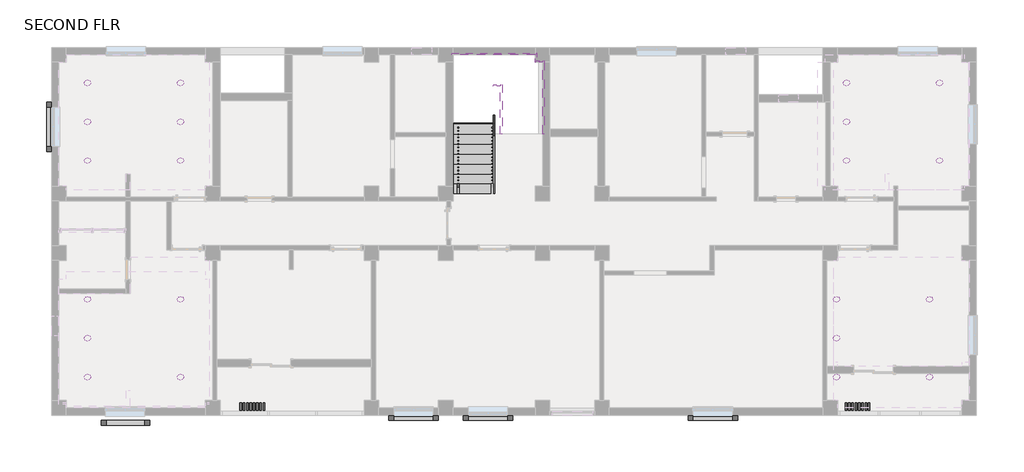
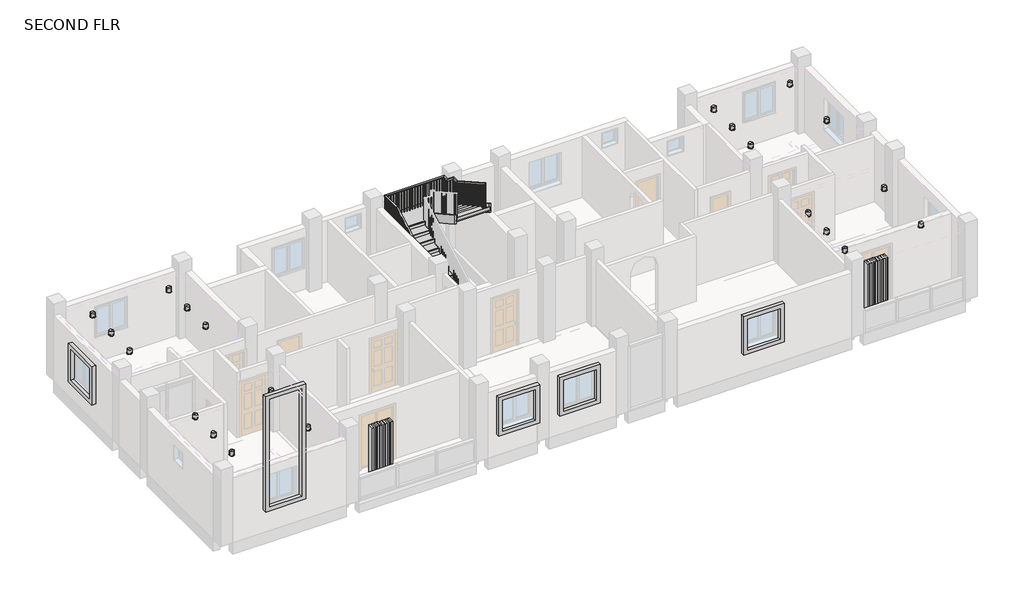
# One storey, part 5 of 5: 21 light fixtures, 8 members, 7 proxies, 1 railing, 1 stair flight.
"""IFC4 building model written with IfcOpenShell, lengths in millimetres."""

from ifc_helpers import new_model, si_unit, frame, origin, place, context, project, spatial, polyline, outline, extrude, faceted_brep, transform, mapped, element, save
from components import generic_models_13_generic_models_7_57cb182b, generic_models_17_generic_models_17_4194431e, generic_models_2_generic_models_2_798ec4a6, generic_models_21_generic_models_21_07dc1754, light_modern_pendant_14774_baffle_cc9af11b, light_modern_pendant_14774_baffle_b3430626, stair_flight_991562f7

model = new_model("IFC4")

# Units and contexts
model_context = context("Model", 3, world=origin())
ifc_project = project(units=[si_unit("LENGTHUNIT", "METRE", prefix="MILLI")], contexts=[model_context])

# Site, building, storey
site = spatial("IfcSite", under=ifc_project)
building = spatial("IfcBuilding", under=site)
storey = spatial("IfcBuildingStorey", under=building, Name="SECOND FLR", Elevation=6400.8)

# Proxies
placement = place(None, origin())
generic_models_13_generic_models_7_shape = generic_models_13_generic_models_7_57cb182b(model_context)
element("IfcBuildingElementProxy", 1, Name="Generic Models 13 : Generic Models 7", ObjectType="Generic Models 13 : Generic Models 7", at=placement, inside=storey, context=model_context, shape_type="MappedRepresentation", body=[
    mapped(generic_models_13_generic_models_7_shape, transform((18592.8, 152.4, 0.0), x_axis=(1.0, 0.0, 0.0), y_axis=(0.0, 1.0, 0.0), z_axis=(0.0, 0.0, 1.0))),
])
generic_models_17_generic_models_17_shape = generic_models_17_generic_models_17_4194431e(model_context)
element("IfcBuildingElementProxy", 2, Name="Generic Models 18 : Generic Models 17", ObjectType="Generic Models 18 : Generic Models 17", at=placement, inside=storey, context=model_context, shape_type="MappedRepresentation", body=[
    mapped(generic_models_17_generic_models_17_shape, transform((0.0, 0.0, -3048.0), x_axis=(1.0, 0.0, 0.0), y_axis=(0.0, 1.0, 0.0), z_axis=(0.0, 0.0, 1.0))),
])
generic_models_2_generic_models_2_shape = generic_models_2_generic_models_2_798ec4a6(model_context)
element("IfcBuildingElementProxy", 3, Name="Generic Models 2 : Generic Models 2", ObjectType="Generic Models 2 : Generic Models 2", at=placement, inside=storey, context=model_context, shape_type="MappedRepresentation", body=[
    mapped(generic_models_2_generic_models_2_shape, transform((0.0, 0.0, 0.0), x_axis=(1.0, 0.0, 0.0), y_axis=(0.0, 1.0, 0.0), z_axis=(0.0, 0.0, 1.0))),
])
generic_models_21_generic_models_21_shape = generic_models_21_generic_models_21_07dc1754(model_context)
element("IfcBuildingElementProxy", 4, Name="Generic Models 22 : Generic Models 21", ObjectType="Generic Models 22 : Generic Models 21", at=placement, inside=storey, context=model_context, shape_type="MappedRepresentation", body=[
    mapped(generic_models_21_generic_models_21_shape, transform((0.0, 0.0, -3048.0), x_axis=(1.0, 0.0, 0.0), y_axis=(0.0, 1.0, 0.0), z_axis=(0.0, 0.0, 1.0))),
])
element("IfcBuildingElementProxy", 5, Name="Generic Models 26 : Generic Models 21", ObjectType="Generic Models 26 : Generic Models 21", at=placement, inside=storey, context=model_context, shape_type="MappedRepresentation", body=[
    mapped(generic_models_21_generic_models_21_shape, transform((-6905.3372689, 0.0, -3048.0), x_axis=(1.0, 0.0, 0.0), y_axis=(0.0, 1.0, 0.0), z_axis=(0.0, 0.0, 1.0))),
])
element("IfcBuildingElementProxy", 6, Name="Generic Models 30 : Generic Models 21", ObjectType="Generic Models 30 : Generic Models 21", at=placement, inside=storey, context=model_context, shape_type="MappedRepresentation", body=[
    mapped(generic_models_21_generic_models_21_shape, transform((-9191.3372689, 0.0, -3048.0), x_axis=(1.0, 0.0, 0.0), y_axis=(0.0, 1.0, 0.0), z_axis=(0.0, 0.0, 1.0))),
])
element("IfcBuildingElementProxy", 7, Name="Generic Models 7 : Generic Models 7", ObjectType="Generic Models 7 : Generic Models 7", at=placement, inside=storey, context=model_context, shape_type="MappedRepresentation", body=[
    mapped(generic_models_13_generic_models_7_shape, transform((0.0, 152.4, 0.0), x_axis=(1.0, 0.0, 0.0), y_axis=(0.0, 1.0, 0.0), z_axis=(0.0, 0.0, 1.0))),
])

# Light fixtures
light_modern_pendant_14774_baffle_shape = light_modern_pendant_14774_baffle_cc9af11b(model_context)
element("IfcLightFixture", 8, ObjectType="LIGHT_-_MODERN_PENDANT_14774 : Baffle", at=placement, inside=storey, context=model_context, shape_type="MappedRepresentation", body=[
    mapped(light_modern_pendant_14774_baffle_shape, transform((-14269.0456086, -897.3794704, 6527.8), x_axis=(1.0, 0.0, 0.0), y_axis=(0.0, 1.0, 0.0), z_axis=(0.0, 0.0, 1.0))),
])
element("IfcLightFixture", 9, ObjectType="LIGHT_-_MODERN_PENDANT_14774 : Baffle", at=placement, inside=storey, context=model_context, shape_type="MappedRepresentation", body=[
    mapped(light_modern_pendant_14774_baffle_shape, transform((-14269.0456086, -3284.9794704, 6527.8), x_axis=(1.0, 0.0, 0.0), y_axis=(0.0, 1.0, 0.0), z_axis=(0.0, 0.0, 1.0))),
])
element("IfcLightFixture", 10, ObjectType="LIGHT_-_MODERN_PENDANT_14774 : Baffle", at=placement, inside=storey, context=model_context, shape_type="MappedRepresentation", body=[
    mapped(light_modern_pendant_14774_baffle_shape, transform((-14269.0456086, -2091.1794704, 6527.8), x_axis=(1.0, 0.0, 0.0), y_axis=(0.0, 1.0, 0.0), z_axis=(0.0, 0.0, 1.0))),
])
element("IfcLightFixture", 11, ObjectType="LIGHT_-_MODERN_PENDANT_14774 : Baffle", at=placement, inside=storey, context=model_context, shape_type="MappedRepresentation", body=[
    mapped(light_modern_pendant_14774_baffle_shape, transform((9048.1543914, -897.3794704, 6527.8), x_axis=(1.0, 0.0, 0.0), y_axis=(0.0, 1.0, 0.0), z_axis=(0.0, 0.0, 1.0))),
])
element("IfcLightFixture", 12, ObjectType="LIGHT_-_MODERN_PENDANT_14774 : Baffle", at=placement, inside=storey, context=model_context, shape_type="MappedRepresentation", body=[
    mapped(light_modern_pendant_14774_baffle_shape, transform((9048.1543914, -3284.9794704, 6527.8), x_axis=(1.0, 0.0, 0.0), y_axis=(0.0, 1.0, 0.0), z_axis=(0.0, 0.0, 1.0))),
])
element("IfcLightFixture", 13, ObjectType="LIGHT_-_MODERN_PENDANT_14774 : Baffle", at=placement, inside=storey, context=model_context, shape_type="MappedRepresentation", body=[
    mapped(light_modern_pendant_14774_baffle_shape, transform((9048.1543914, -2091.1794704, 6527.8), x_axis=(1.0, 0.0, 0.0), y_axis=(0.0, 1.0, 0.0), z_axis=(0.0, 0.0, 1.0))),
])
element("IfcLightFixture", 14, ObjectType="LIGHT_-_MODERN_PENDANT_14774 : Baffle", at=placement, inside=storey, context=model_context, shape_type="MappedRepresentation", body=[
    mapped(light_modern_pendant_14774_baffle_shape, transform((-14269.0456086, -7552.1794704, 6527.8), x_axis=(1.0, 0.0, 0.0), y_axis=(0.0, 1.0, 0.0), z_axis=(0.0, 0.0, 1.0))),
])
element("IfcLightFixture", 15, ObjectType="LIGHT_-_MODERN_PENDANT_14774 : Baffle", at=placement, inside=storey, context=model_context, shape_type="MappedRepresentation", body=[
    mapped(light_modern_pendant_14774_baffle_shape, transform((-14269.0456086, -9939.7794704, 6527.8), x_axis=(1.0, 0.0, 0.0), y_axis=(0.0, 1.0, 0.0), z_axis=(0.0, 0.0, 1.0))),
])
element("IfcLightFixture", 16, ObjectType="LIGHT_-_MODERN_PENDANT_14774 : Baffle", at=placement, inside=storey, context=model_context, shape_type="MappedRepresentation", body=[
    mapped(light_modern_pendant_14774_baffle_shape, transform((-14269.0456086, -8745.9794704, 6527.8), x_axis=(1.0, 0.0, 0.0), y_axis=(0.0, 1.0, 0.0), z_axis=(0.0, 0.0, 1.0))),
])
element("IfcLightFixture", 17, ObjectType="LIGHT_-_MODERN_PENDANT_14774 : Baffle", at=placement, inside=storey, context=model_context, shape_type="MappedRepresentation", body=[
    mapped(light_modern_pendant_14774_baffle_shape, transform((8743.3543914, -7552.1794704, 6527.8), x_axis=(1.0, 0.0, 0.0), y_axis=(0.0, 1.0, 0.0), z_axis=(0.0, 0.0, 1.0))),
])
element("IfcLightFixture", 18, ObjectType="LIGHT_-_MODERN_PENDANT_14774 : Baffle", at=placement, inside=storey, context=model_context, shape_type="MappedRepresentation", body=[
    mapped(light_modern_pendant_14774_baffle_shape, transform((8743.3543914, -9939.7794704, 6527.8), x_axis=(1.0, 0.0, 0.0), y_axis=(0.0, 1.0, 0.0), z_axis=(0.0, 0.0, 1.0))),
])
element("IfcLightFixture", 19, ObjectType="LIGHT_-_MODERN_PENDANT_14774 : Baffle", at=placement, inside=storey, context=model_context, shape_type="MappedRepresentation", body=[
    mapped(light_modern_pendant_14774_baffle_shape, transform((8743.3543914, -8745.9794704, 6527.8), x_axis=(1.0, 0.0, 0.0), y_axis=(0.0, 1.0, 0.0), z_axis=(0.0, 0.0, 1.0))),
])
light_modern_pendant_14774_baffle_2_shape = light_modern_pendant_14774_baffle_b3430626(model_context)
element("IfcLightFixture", 20, ObjectType="LIGHT_-_MODERN_PENDANT_14774 : Baffle", at=placement, inside=storey, context=model_context, shape_type="MappedRepresentation", body=[
    mapped(light_modern_pendant_14774_baffle_2_shape, transform((-11411.5456086, -897.3794704, 6527.8), x_axis=(-1.0, 0.0, 0.0), y_axis=(0.0, -1.0, 0.0), z_axis=(0.0, 0.0, 1.0))),
])
element("IfcLightFixture", 21, ObjectType="LIGHT_-_MODERN_PENDANT_14774 : Baffle", at=placement, inside=storey, context=model_context, shape_type="MappedRepresentation", body=[
    mapped(light_modern_pendant_14774_baffle_2_shape, transform((-11411.5456086, -3284.9794704, 6527.8), x_axis=(-1.0, 0.0, 0.0), y_axis=(0.0, -1.0, 0.0), z_axis=(0.0, 0.0, 1.0))),
])
element("IfcLightFixture", 22, ObjectType="LIGHT_-_MODERN_PENDANT_14774 : Baffle", at=placement, inside=storey, context=model_context, shape_type="MappedRepresentation", body=[
    mapped(light_modern_pendant_14774_baffle_2_shape, transform((-11411.5456086, -2091.1794704, 6527.8), x_axis=(-1.0, 0.0, 0.0), y_axis=(0.0, -1.0, 0.0), z_axis=(0.0, 0.0, 1.0))),
])
element("IfcLightFixture", 23, ObjectType="LIGHT_-_MODERN_PENDANT_14774 : Baffle", at=placement, inside=storey, context=model_context, shape_type="MappedRepresentation", body=[
    mapped(light_modern_pendant_14774_baffle_2_shape, transform((11905.6543914, -897.3794704, 6527.8), x_axis=(-1.0, 0.0, 0.0), y_axis=(0.0, -1.0, 0.0), z_axis=(0.0, 0.0, 1.0))),
])
element("IfcLightFixture", 24, ObjectType="LIGHT_-_MODERN_PENDANT_14774 : Baffle", at=placement, inside=storey, context=model_context, shape_type="MappedRepresentation", body=[
    mapped(light_modern_pendant_14774_baffle_2_shape, transform((11905.6543914, -3284.9794704, 6527.8), x_axis=(-1.0, 0.0, 0.0), y_axis=(0.0, -1.0, 0.0), z_axis=(0.0, 0.0, 1.0))),
])
element("IfcLightFixture", 25, ObjectType="LIGHT_-_MODERN_PENDANT_14774 : Baffle", at=placement, inside=storey, context=model_context, shape_type="MappedRepresentation", body=[
    mapped(light_modern_pendant_14774_baffle_2_shape, transform((-11411.5456086, -7552.1794704, 6527.8), x_axis=(-1.0, 0.0, 0.0), y_axis=(0.0, -1.0, 0.0), z_axis=(0.0, 0.0, 1.0))),
])
element("IfcLightFixture", 26, ObjectType="LIGHT_-_MODERN_PENDANT_14774 : Baffle", at=placement, inside=storey, context=model_context, shape_type="MappedRepresentation", body=[
    mapped(light_modern_pendant_14774_baffle_2_shape, transform((-11411.5456086, -9939.7794704, 6527.8), x_axis=(-1.0, 0.0, 0.0), y_axis=(0.0, -1.0, 0.0), z_axis=(0.0, 0.0, 1.0))),
])
element("IfcLightFixture", 27, ObjectType="LIGHT_-_MODERN_PENDANT_14774 : Baffle", at=placement, inside=storey, context=model_context, shape_type="MappedRepresentation", body=[
    mapped(light_modern_pendant_14774_baffle_2_shape, transform((11600.8543914, -7552.1794704, 6527.8), x_axis=(-1.0, 0.0, 0.0), y_axis=(0.0, -1.0, 0.0), z_axis=(0.0, 0.0, 1.0))),
])
element("IfcLightFixture", 28, ObjectType="LIGHT_-_MODERN_PENDANT_14774 : Baffle", at=placement, inside=storey, context=model_context, shape_type="MappedRepresentation", body=[
    mapped(light_modern_pendant_14774_baffle_2_shape, transform((11600.8543914, -9939.7794704, 6527.8), x_axis=(-1.0, 0.0, 0.0), y_axis=(0.0, -1.0, 0.0), z_axis=(0.0, 0.0, 1.0))),
])

# Members
element("IfcMember", 29, ObjectType="Stringer - 2\" Width", at=placement, inside=storey, context=model_context, shape_type="SweptSolid", body=[
    extrude(outline(polyline([(-4300.9794704, 6400.8), (-4300.9794704, 6608.3983948), (-879.896581, 8509.0), (-252.2749676, 8509.0), (-4047.0349676, 6400.8), (-4300.9794704, 6400.8)])), frame((-3080.3456086, 0.0, 0.0), z_axis=(1.0, 0.0, 0.0), x_axis=(0.0, 1.0, 0.0)), (0.0, 0.0, 1.0), 50.8),
])
element("IfcMember", 30, ObjectType="Stringer - 2\" Width", at=placement, inside=storey, context=model_context, shape_type="SweptSolid", body=[
    extrude(outline(polyline([(-3080.3456086, -33.7794704), (-3080.3456086, 17.0205296), (-467.6083398, 17.0205296), (-518.4083398, -33.7794704), (-3080.3456086, -33.7794704)])), frame((0.0, 0.0, 8204.2), z_axis=(0.0, 0.0, 1.0), x_axis=(1.0, 0.0, 0.0)), (0.0, 0.0, 1.0), 304.8),
])
element("IfcMember", 31, ObjectType="Stringer - 2\" Width", at=placement, inside=storey, context=model_context, shape_type="SweptSolid", body=[
    extrude(outline(polyline([(-518.4083398, -33.7794704), (-467.6083398, 17.0205296), (-467.6083398, -211.5794704), (-518.4083398, -262.3794704), (-518.4083398, -33.7794704)])), frame((0.0, 0.0, 8204.2), z_axis=(0.0, 0.0, 1.0), x_axis=(1.0, 0.0, 0.0)), (0.0, 0.0, 1.0), 304.8),
])
element("IfcMember", 32, ObjectType="Stringer - 2\" Width", at=placement, inside=storey, context=model_context, shape_type="SweptSolid", body=[
    extrude(outline(polyline([(-518.4083398, -262.3794704), (-467.6083398, -211.5794704), (-289.8083398, -211.5794704), (-289.8083398, -262.3794704), (-518.4083398, -262.3794704)])), frame((0.0, 0.0, 8204.2), z_axis=(0.0, 0.0, 1.0), x_axis=(1.0, 0.0, 0.0)), (0.0, 0.0, 1.0), 304.8),
])
element("IfcMember", 33, ObjectType="Stringer - 2\" Width", at=placement, inside=storey, context=model_context, shape_type="SweptSolid", body=[
    extrude(outline(polyline([(-211.5794704, 8231.1761726), (-211.5794704, 8204.2), (-790.6439732, 8204.2), (-2472.1794704, 9138.3863873), (-2472.1794704, 9487.0650614), (-211.5794704, 8231.1761726)])), frame((-289.8083398, 0.0, 0.0), z_axis=(1.0, 0.0, 0.0), x_axis=(0.0, 1.0, 0.0)), (0.0, 0.0, 1.0), 50.8),
])
element("IfcMember", 34, ObjectType="Stringer - 2\" Width", at=placement, inside=storey, context=model_context, shape_type="SweptSolid", body=[
    extrude(outline(polyline([(-4300.9794704, 6400.8), (-4300.9794704, 6608.3983948), (-998.9794704, 8442.8428392), (-998.9794704, 8094.1641651), (-4047.0349676, 6400.8), (-4300.9794704, 6400.8)])), frame((-1810.3456086, 0.0, 0.0), z_axis=(1.0, 0.0, 0.0), x_axis=(0.0, 1.0, 0.0)), (0.0, 0.0, 1.0), 50.8),
])
element("IfcMember", 35, ObjectType="Stringer - 2\" Width", at=placement, inside=storey, context=model_context, shape_type="SweptSolid", body=[
    extrude(outline(polyline([(-1810.3456086, -998.9794704), (-1810.3456086, -948.1794704), (-1585.2083398, -948.1794704), (-1585.2083398, -998.9794704), (-1810.3456086, -998.9794704)])), frame((0.0, 0.0, 8204.2), z_axis=(0.0, 0.0, 1.0), x_axis=(1.0, 0.0, 0.0)), (0.0, 0.0, 1.0), 304.8),
])
element("IfcMember", 36, ObjectType="Stringer - 2\" Width", at=placement, inside=storey, context=model_context, shape_type="SweptSolid", body=[
    extrude(outline(polyline([(-948.1794704, 8640.3983948), (-948.1794704, 8291.7197207), (-2472.1794704, 9138.3863873), (-2472.1794704, 9487.0650614), (-948.1794704, 8640.3983948)])), frame((-1585.2083398, 0.0, 0.0), z_axis=(1.0, 0.0, 0.0), x_axis=(0.0, 1.0, 0.0)), (0.0, 0.0, 1.0), 50.8),
])

# Railing
element("IfcRailing", 37, ObjectType="Handrail - Rectangular", at=placement, inside=storey, context=model_context, shape_type="SolidModel", body=[
    faceted_brep([(-2902.5456086, -4300.9794704, 7484.5333333), (-2902.5456086, -4300.9794704, 7426.420221), (-2851.7456086, -4300.9794704, 7426.420221), (-2851.7456086, -4300.9794704, 7484.5333333), (-2902.5456086, -948.1794704, 9347.2), (-2902.5456086, -935.0158682, 9296.4), (-2851.7456086, -935.0158682, 9296.4), (-2851.7456086, -948.1794704, 9347.2), (-2902.5456086, -160.7794704, 9347.2), (-2902.5456086, -160.7794704, 9296.4), (-2851.7456086, -211.5794704, 9296.4), (-2851.7456086, -211.5794704, 9347.2), (-645.4083398, -160.7794704, 9347.2), (-645.4083398, -160.7794704, 9296.4), (-696.2083398, -211.5794704, 9296.4), (-696.2083398, -211.5794704, 9347.2), (-645.4083398, -389.3794704, 9347.2), (-645.4083398, -389.3794704, 9296.4), (-696.2083398, -440.1794704, 9296.4), (-696.2083398, -440.1794704, 9347.2), (-416.8083398, -389.3794704, 9347.2), (-416.8083398, -389.3794704, 9296.4), (-467.6083398, -440.1794704, 9296.4), (-467.6083398, -440.1794704, 9347.2), (-416.8083398, -643.3794704, 9347.2), (-416.8083398, -656.5430727, 9296.4), (-467.6083398, -656.5430727, 9296.4), (-467.6083398, -643.3794704, 9347.2), (-416.8083398, -2472.1794704, 10363.2), (-467.6083398, -2472.1794704, 10363.2), (-467.6083398, -2472.1794704, 10305.0868876), (-416.8083398, -2472.1794704, 10305.0868876)], [[[0, 1, 2, 3]], [[1, 0, 4, 5]], [[2, 1, 5, 6]], [[3, 2, 6, 7]], [[0, 3, 7, 4]], [[5, 4, 8, 9]], [[6, 5, 9, 10]], [[7, 6, 10, 11]], [[4, 7, 11, 8]], [[9, 8, 12, 13]], [[10, 9, 13, 14]], [[11, 10, 14, 15]], [[8, 11, 15, 12]], [[13, 12, 16, 17]], [[14, 13, 17, 18]], [[15, 14, 18, 19]], [[12, 15, 19, 16]], [[17, 16, 20, 21]], [[18, 17, 21, 22]], [[19, 18, 22, 23]], [[16, 19, 23, 20]], [[21, 20, 24, 25]], [[22, 21, 25, 26]], [[23, 22, 26, 27]], [[20, 23, 27, 24]], [[28, 29, 30, 31]], [[25, 24, 28, 31]], [[26, 25, 31, 30]], [[27, 26, 30, 29]], [[24, 27, 29, 28]]]),
    extrude(outline(polyline([(-2437.2544704, 10285.6841099), (-2437.2544704, 9279.4666667), (-2456.3044704, 9279.4666667), (-2456.3044704, 10296.2674432), (-2437.2544704, 10285.6841099)])), frame((-451.7333398, 0.0, 0.0), z_axis=(1.0, 0.0, 0.0), x_axis=(0.0, 1.0, 0.0)), (0.0, 0.0, 1.0), 19.05),
    extrude(outline(polyline([(-2335.6544704, 10229.2396654), (-2335.6544704, 9279.4666667), (-2354.7044704, 9279.4666667), (-2354.7044704, 10239.8229988), (-2335.6544704, 10229.2396654)])), frame((-451.7333398, 0.0, 0.0), z_axis=(1.0, 0.0, 0.0), x_axis=(0.0, 1.0, 0.0)), (0.0, 0.0, 1.0), 19.05),
    extrude(outline(polyline([(-2234.0544704, 10172.795221), (-2234.0544704, 9279.4666667), (-2253.1044704, 9279.4666667), (-2253.1044704, 10183.3785543), (-2234.0544704, 10172.795221)])), frame((-451.7333398, 0.0, 0.0), z_axis=(1.0, 0.0, 0.0), x_axis=(0.0, 1.0, 0.0)), (0.0, 0.0, 1.0), 19.05),
    extrude(outline(polyline([(-2132.4544704, 10116.3507765), (-2132.4544704, 9110.1333333), (-2151.5044704, 9110.1333333), (-2151.5044704, 10126.9341099), (-2132.4544704, 10116.3507765)])), frame((-451.7333398, 0.0, 0.0), z_axis=(1.0, 0.0, 0.0), x_axis=(0.0, 1.0, 0.0)), (0.0, 0.0, 1.0), 19.05),
    extrude(outline(polyline([(-2030.8544704, 10059.9063321), (-2030.8544704, 9110.1333333), (-2049.9044704, 9110.1333333), (-2049.9044704, 10070.4896654), (-2030.8544704, 10059.9063321)])), frame((-451.7333398, 0.0, 0.0), z_axis=(1.0, 0.0, 0.0), x_axis=(0.0, 1.0, 0.0)), (0.0, 0.0, 1.0), 19.05),
    extrude(outline(polyline([(-1929.2544704, 10003.4618876), (-1929.2544704, 9110.1333333), (-1948.3044704, 9110.1333333), (-1948.3044704, 10014.045221), (-1929.2544704, 10003.4618876)])), frame((-451.7333398, 0.0, 0.0), z_axis=(1.0, 0.0, 0.0), x_axis=(0.0, 1.0, 0.0)), (0.0, 0.0, 1.0), 19.05),
    extrude(outline(polyline([(-1827.6544704, 9947.0174432), (-1827.6544704, 8940.8), (-1846.7044704, 8940.8), (-1846.7044704, 9957.6007765), (-1827.6544704, 9947.0174432)])), frame((-451.7333398, 0.0, 0.0), z_axis=(1.0, 0.0, 0.0), x_axis=(0.0, 1.0, 0.0)), (0.0, 0.0, 1.0), 19.05),
    extrude(outline(polyline([(-1726.0544704, 9890.5729988), (-1726.0544704, 8940.8), (-1745.1044704, 8940.8), (-1745.1044704, 9901.1563321), (-1726.0544704, 9890.5729988)])), frame((-451.7333398, 0.0, 0.0), z_axis=(1.0, 0.0, 0.0), x_axis=(0.0, 1.0, 0.0)), (0.0, 0.0, 1.0), 19.05),
    extrude(outline(polyline([(-1624.4544704, 9834.1285543), (-1624.4544704, 8940.8), (-1643.5044704, 8940.8), (-1643.5044704, 9844.7118876), (-1624.4544704, 9834.1285543)])), frame((-451.7333398, 0.0, 0.0), z_axis=(1.0, 0.0, 0.0), x_axis=(0.0, 1.0, 0.0)), (0.0, 0.0, 1.0), 19.05),
    extrude(outline(polyline([(-1522.8544704, 9777.6841099), (-1522.8544704, 8771.4666667), (-1541.9044704, 8771.4666667), (-1541.9044704, 9788.2674432), (-1522.8544704, 9777.6841099)])), frame((-451.7333398, 0.0, 0.0), z_axis=(1.0, 0.0, 0.0), x_axis=(0.0, 1.0, 0.0)), (0.0, 0.0, 1.0), 19.05),
    extrude(outline(polyline([(-1421.2544704, 9721.2396654), (-1421.2544704, 8771.4666667), (-1440.3044704, 8771.4666667), (-1440.3044704, 9731.8229988), (-1421.2544704, 9721.2396654)])), frame((-451.7333398, 0.0, 0.0), z_axis=(1.0, 0.0, 0.0), x_axis=(0.0, 1.0, 0.0)), (0.0, 0.0, 1.0), 19.05),
    extrude(outline(polyline([(-1319.6544704, 9664.795221), (-1319.6544704, 8771.4666667), (-1338.7044704, 8771.4666667), (-1338.7044704, 9675.3785543), (-1319.6544704, 9664.795221)])), frame((-451.7333398, 0.0, 0.0), z_axis=(1.0, 0.0, 0.0), x_axis=(0.0, 1.0, 0.0)), (0.0, 0.0, 1.0), 19.05),
    extrude(outline(polyline([(-1218.0544704, 9608.3507765), (-1218.0544704, 8602.1333333), (-1237.1044704, 8602.1333333), (-1237.1044704, 9618.9341099), (-1218.0544704, 9608.3507765)])), frame((-451.7333398, 0.0, 0.0), z_axis=(1.0, 0.0, 0.0), x_axis=(0.0, 1.0, 0.0)), (0.0, 0.0, 1.0), 19.05),
    extrude(outline(polyline([(-1116.4544704, 9551.9063321), (-1116.4544704, 8602.1333333), (-1135.5044704, 8602.1333333), (-1135.5044704, 9562.4896654), (-1116.4544704, 9551.9063321)])), frame((-451.7333398, 0.0, 0.0), z_axis=(1.0, 0.0, 0.0), x_axis=(0.0, 1.0, 0.0)), (0.0, 0.0, 1.0), 19.05),
    extrude(outline(polyline([(-1014.8544704, 9495.4618876), (-1014.8544704, 8602.1333333), (-1033.9044704, 8602.1333333), (-1033.9044704, 9506.045221), (-1014.8544704, 9495.4618876)])), frame((-451.7333398, 0.0, 0.0), z_axis=(1.0, 0.0, 0.0), x_axis=(0.0, 1.0, 0.0)), (0.0, 0.0, 1.0), 19.05),
    extrude(outline(polyline([(-913.2544704, 9439.0174432), (-913.2544704, 8432.8), (-932.3044704, 8432.8), (-932.3044704, 9449.6007765), (-913.2544704, 9439.0174432)])), frame((-451.7333398, 0.0, 0.0), z_axis=(1.0, 0.0, 0.0), x_axis=(0.0, 1.0, 0.0)), (0.0, 0.0, 1.0), 19.05),
    extrude(outline(polyline([(-811.6544704, 9382.5729988), (-811.6544704, 8432.8), (-830.7044704, 8432.8), (-830.7044704, 9393.1563321), (-811.6544704, 9382.5729988)])), frame((-451.7333398, 0.0, 0.0), z_axis=(1.0, 0.0, 0.0), x_axis=(0.0, 1.0, 0.0)), (0.0, 0.0, 1.0), 19.05),
    extrude(outline(polyline([(-710.0544704, 9326.1285543), (-710.0544704, 8432.8), (-729.1044704, 8432.8), (-729.1044704, 9336.7118876), (-710.0544704, 9326.1285543)])), frame((-451.7333398, 0.0, 0.0), z_axis=(1.0, 0.0, 0.0), x_axis=(0.0, 1.0, 0.0)), (0.0, 0.0, 1.0), 19.05),
    extrude(outline(polyline([(-432.6833398, -608.4544704), (-432.6833398, -627.5044704), (-451.7333398, -627.5044704), (-451.7333398, -608.4544704), (-432.6833398, -608.4544704)])), frame((0.0, 0.0, 8432.8), z_axis=(0.0, 0.0, 1.0), x_axis=(1.0, 0.0, 0.0)), (0.0, 0.0, 1.0), 863.6),
    extrude(outline(polyline([(-432.6833398, -506.8544704), (-432.6833398, -525.9044704), (-451.7333398, -525.9044704), (-451.7333398, -506.8544704), (-432.6833398, -506.8544704)])), frame((0.0, 0.0, 8432.8), z_axis=(0.0, 0.0, 1.0), x_axis=(1.0, 0.0, 0.0)), (0.0, 0.0, 1.0), 863.6),
    extrude(outline(polyline([(-477.1333398, -405.2544704), (-458.0833398, -405.2544704), (-458.0833398, -424.3044704), (-477.1333398, -424.3044704), (-477.1333398, -405.2544704)])), frame((0.0, 0.0, 8432.8), z_axis=(0.0, 0.0, 1.0), x_axis=(1.0, 0.0, 0.0)), (0.0, 0.0, 1.0), 863.6),
    extrude(outline(polyline([(-578.7333398, -405.2544704), (-559.6833398, -405.2544704), (-559.6833398, -424.3044704), (-578.7333398, -424.3044704), (-578.7333398, -405.2544704)])), frame((0.0, 0.0, 8432.8), z_axis=(0.0, 0.0, 1.0), x_axis=(1.0, 0.0, 0.0)), (0.0, 0.0, 1.0), 863.6),
    extrude(outline(polyline([(-661.2833398, -379.8544704), (-661.2833398, -398.9044704), (-680.3333398, -398.9044704), (-680.3333398, -379.8544704), (-661.2833398, -379.8544704)])), frame((0.0, 0.0, 8432.8), z_axis=(0.0, 0.0, 1.0), x_axis=(1.0, 0.0, 0.0)), (0.0, 0.0, 1.0), 863.6),
    extrude(outline(polyline([(-661.2833398, -278.2544704), (-661.2833398, -297.3044704), (-680.3333398, -297.3044704), (-680.3333398, -278.2544704), (-661.2833398, -278.2544704)])), frame((0.0, 0.0, 8432.8), z_axis=(0.0, 0.0, 1.0), x_axis=(1.0, 0.0, 0.0)), (0.0, 0.0, 1.0), 863.6),
    extrude(outline(polyline([(-753.0706086, -176.6544704), (-734.0206086, -176.6544704), (-734.0206086, -195.7044704), (-753.0706086, -195.7044704), (-753.0706086, -176.6544704)])), frame((0.0, 0.0, 8432.8), z_axis=(0.0, 0.0, 1.0), x_axis=(1.0, 0.0, 0.0)), (0.0, 0.0, 1.0), 863.6),
    extrude(outline(polyline([(-854.6706086, -176.6544704), (-835.6206086, -176.6544704), (-835.6206086, -195.7044704), (-854.6706086, -195.7044704), (-854.6706086, -176.6544704)])), frame((0.0, 0.0, 8432.8), z_axis=(0.0, 0.0, 1.0), x_axis=(1.0, 0.0, 0.0)), (0.0, 0.0, 1.0), 863.6),
    extrude(outline(polyline([(-956.2706086, -176.6544704), (-937.2206086, -176.6544704), (-937.2206086, -195.7044704), (-956.2706086, -195.7044704), (-956.2706086, -176.6544704)])), frame((0.0, 0.0, 8432.8), z_axis=(0.0, 0.0, 1.0), x_axis=(1.0, 0.0, 0.0)), (0.0, 0.0, 1.0), 863.6),
    extrude(outline(polyline([(-1057.8706086, -176.6544704), (-1038.8206086, -176.6544704), (-1038.8206086, -195.7044704), (-1057.8706086, -195.7044704), (-1057.8706086, -176.6544704)])), frame((0.0, 0.0, 8432.8), z_axis=(0.0, 0.0, 1.0), x_axis=(1.0, 0.0, 0.0)), (0.0, 0.0, 1.0), 863.6),
    extrude(outline(polyline([(-1159.4706086, -176.6544704), (-1140.4206086, -176.6544704), (-1140.4206086, -195.7044704), (-1159.4706086, -195.7044704), (-1159.4706086, -176.6544704)])), frame((0.0, 0.0, 8432.8), z_axis=(0.0, 0.0, 1.0), x_axis=(1.0, 0.0, 0.0)), (0.0, 0.0, 1.0), 863.6),
    extrude(outline(polyline([(-1261.0706086, -176.6544704), (-1242.0206086, -176.6544704), (-1242.0206086, -195.7044704), (-1261.0706086, -195.7044704), (-1261.0706086, -176.6544704)])), frame((0.0, 0.0, 8432.8), z_axis=(0.0, 0.0, 1.0), x_axis=(1.0, 0.0, 0.0)), (0.0, 0.0, 1.0), 863.6),
    extrude(outline(polyline([(-1362.6706086, -176.6544704), (-1343.6206086, -176.6544704), (-1343.6206086, -195.7044704), (-1362.6706086, -195.7044704), (-1362.6706086, -176.6544704)])), frame((0.0, 0.0, 8432.8), z_axis=(0.0, 0.0, 1.0), x_axis=(1.0, 0.0, 0.0)), (0.0, 0.0, 1.0), 863.6),
    extrude(outline(polyline([(-1464.2706086, -176.6544704), (-1445.2206086, -176.6544704), (-1445.2206086, -195.7044704), (-1464.2706086, -195.7044704), (-1464.2706086, -176.6544704)])), frame((0.0, 0.0, 8432.8), z_axis=(0.0, 0.0, 1.0), x_axis=(1.0, 0.0, 0.0)), (0.0, 0.0, 1.0), 863.6),
    extrude(outline(polyline([(-1565.8706086, -176.6544704), (-1546.8206086, -176.6544704), (-1546.8206086, -195.7044704), (-1565.8706086, -195.7044704), (-1565.8706086, -176.6544704)])), frame((0.0, 0.0, 8432.8), z_axis=(0.0, 0.0, 1.0), x_axis=(1.0, 0.0, 0.0)), (0.0, 0.0, 1.0), 863.6),
    extrude(outline(polyline([(-1667.4706086, -176.6544704), (-1648.4206086, -176.6544704), (-1648.4206086, -195.7044704), (-1667.4706086, -195.7044704), (-1667.4706086, -176.6544704)])), frame((0.0, 0.0, 8432.8), z_axis=(0.0, 0.0, 1.0), x_axis=(1.0, 0.0, 0.0)), (0.0, 0.0, 1.0), 863.6),
    extrude(outline(polyline([(-1769.0706086, -176.6544704), (-1750.0206086, -176.6544704), (-1750.0206086, -195.7044704), (-1769.0706086, -195.7044704), (-1769.0706086, -176.6544704)])), frame((0.0, 0.0, 8432.8), z_axis=(0.0, 0.0, 1.0), x_axis=(1.0, 0.0, 0.0)), (0.0, 0.0, 1.0), 863.6),
    extrude(outline(polyline([(-1870.6706086, -176.6544704), (-1851.6206086, -176.6544704), (-1851.6206086, -195.7044704), (-1870.6706086, -195.7044704), (-1870.6706086, -176.6544704)])), frame((0.0, 0.0, 8432.8), z_axis=(0.0, 0.0, 1.0), x_axis=(1.0, 0.0, 0.0)), (0.0, 0.0, 1.0), 863.6),
    extrude(outline(polyline([(-1972.2706086, -176.6544704), (-1953.2206086, -176.6544704), (-1953.2206086, -195.7044704), (-1972.2706086, -195.7044704), (-1972.2706086, -176.6544704)])), frame((0.0, 0.0, 8432.8), z_axis=(0.0, 0.0, 1.0), x_axis=(1.0, 0.0, 0.0)), (0.0, 0.0, 1.0), 863.6),
    extrude(outline(polyline([(-2073.8706086, -176.6544704), (-2054.8206086, -176.6544704), (-2054.8206086, -195.7044704), (-2073.8706086, -195.7044704), (-2073.8706086, -176.6544704)])), frame((0.0, 0.0, 8432.8), z_axis=(0.0, 0.0, 1.0), x_axis=(1.0, 0.0, 0.0)), (0.0, 0.0, 1.0), 863.6),
    extrude(outline(polyline([(-2175.4706086, -176.6544704), (-2156.4206086, -176.6544704), (-2156.4206086, -195.7044704), (-2175.4706086, -195.7044704), (-2175.4706086, -176.6544704)])), frame((0.0, 0.0, 8432.8), z_axis=(0.0, 0.0, 1.0), x_axis=(1.0, 0.0, 0.0)), (0.0, 0.0, 1.0), 863.6),
    extrude(outline(polyline([(-2277.0706086, -176.6544704), (-2258.0206086, -176.6544704), (-2258.0206086, -195.7044704), (-2277.0706086, -195.7044704), (-2277.0706086, -176.6544704)])), frame((0.0, 0.0, 8432.8), z_axis=(0.0, 0.0, 1.0), x_axis=(1.0, 0.0, 0.0)), (0.0, 0.0, 1.0), 863.6),
    extrude(outline(polyline([(-2378.6706086, -176.6544704), (-2359.6206086, -176.6544704), (-2359.6206086, -195.7044704), (-2378.6706086, -195.7044704), (-2378.6706086, -176.6544704)])), frame((0.0, 0.0, 8432.8), z_axis=(0.0, 0.0, 1.0), x_axis=(1.0, 0.0, 0.0)), (0.0, 0.0, 1.0), 863.6),
    extrude(outline(polyline([(-2480.2706086, -176.6544704), (-2461.2206086, -176.6544704), (-2461.2206086, -195.7044704), (-2480.2706086, -195.7044704), (-2480.2706086, -176.6544704)])), frame((0.0, 0.0, 8432.8), z_axis=(0.0, 0.0, 1.0), x_axis=(1.0, 0.0, 0.0)), (0.0, 0.0, 1.0), 863.6),
    extrude(outline(polyline([(-2581.8706086, -176.6544704), (-2562.8206086, -176.6544704), (-2562.8206086, -195.7044704), (-2581.8706086, -195.7044704), (-2581.8706086, -176.6544704)])), frame((0.0, 0.0, 8432.8), z_axis=(0.0, 0.0, 1.0), x_axis=(1.0, 0.0, 0.0)), (0.0, 0.0, 1.0), 863.6),
    extrude(outline(polyline([(-2683.4706086, -176.6544704), (-2664.4206086, -176.6544704), (-2664.4206086, -195.7044704), (-2683.4706086, -195.7044704), (-2683.4706086, -176.6544704)])), frame((0.0, 0.0, 8432.8), z_axis=(0.0, 0.0, 1.0), x_axis=(1.0, 0.0, 0.0)), (0.0, 0.0, 1.0), 863.6),
    extrude(outline(polyline([(-2785.0706086, -176.6544704), (-2766.0206086, -176.6544704), (-2766.0206086, -195.7044704), (-2785.0706086, -195.7044704), (-2785.0706086, -176.6544704)])), frame((0.0, 0.0, 8432.8), z_axis=(0.0, 0.0, 1.0), x_axis=(1.0, 0.0, 0.0)), (0.0, 0.0, 1.0), 863.6),
    extrude(outline(polyline([(-2886.6706086, -246.5044704), (-2886.6706086, -227.4544704), (-2867.6206086, -227.4544704), (-2867.6206086, -246.5044704), (-2886.6706086, -246.5044704)])), frame((0.0, 0.0, 8432.8), z_axis=(0.0, 0.0, 1.0), x_axis=(1.0, 0.0, 0.0)), (0.0, 0.0, 1.0), 863.6),
    extrude(outline(polyline([(-2886.6706086, -348.1044704), (-2886.6706086, -329.0544704), (-2867.6206086, -329.0544704), (-2867.6206086, -348.1044704), (-2886.6706086, -348.1044704)])), frame((0.0, 0.0, 8432.8), z_axis=(0.0, 0.0, 1.0), x_axis=(1.0, 0.0, 0.0)), (0.0, 0.0, 1.0), 863.6),
    extrude(outline(polyline([(-2886.6706086, -449.7044704), (-2886.6706086, -430.6544704), (-2867.6206086, -430.6544704), (-2867.6206086, -449.7044704), (-2886.6706086, -449.7044704)])), frame((0.0, 0.0, 8432.8), z_axis=(0.0, 0.0, 1.0), x_axis=(1.0, 0.0, 0.0)), (0.0, 0.0, 1.0), 863.6),
    extrude(outline(polyline([(-2886.6706086, -551.3044704), (-2886.6706086, -532.2544704), (-2867.6206086, -532.2544704), (-2867.6206086, -551.3044704), (-2886.6706086, -551.3044704)])), frame((0.0, 0.0, 8432.8), z_axis=(0.0, 0.0, 1.0), x_axis=(1.0, 0.0, 0.0)), (0.0, 0.0, 1.0), 863.6),
    extrude(outline(polyline([(-2886.6706086, -652.9044704), (-2886.6706086, -633.8544704), (-2867.6206086, -633.8544704), (-2867.6206086, -652.9044704), (-2886.6706086, -652.9044704)])), frame((0.0, 0.0, 8432.8), z_axis=(0.0, 0.0, 1.0), x_axis=(1.0, 0.0, 0.0)), (0.0, 0.0, 1.0), 863.6),
    extrude(outline(polyline([(-2886.6706086, -754.5044704), (-2886.6706086, -735.4544704), (-2867.6206086, -735.4544704), (-2867.6206086, -754.5044704), (-2886.6706086, -754.5044704)])), frame((0.0, 0.0, 8432.8), z_axis=(0.0, 0.0, 1.0), x_axis=(1.0, 0.0, 0.0)), (0.0, 0.0, 1.0), 863.6),
    extrude(outline(polyline([(-2886.6706086, -856.1044704), (-2886.6706086, -837.0544704), (-2867.6206086, -837.0544704), (-2867.6206086, -856.1044704), (-2886.6706086, -856.1044704)])), frame((0.0, 0.0, 8432.8), z_axis=(0.0, 0.0, 1.0), x_axis=(1.0, 0.0, 0.0)), (0.0, 0.0, 1.0), 863.6),
    extrude(outline(polyline([(-938.6544704, 9294.3785543), (-938.6544704, 8432.8), (-957.7044704, 8432.8), (-957.7044704, 9283.795221), (-938.6544704, 9294.3785543)])), frame((-2886.6706086, 0.0, 0.0), z_axis=(1.0, 0.0, 0.0), x_axis=(0.0, 1.0, 0.0)), (0.0, 0.0, 1.0), 19.05),
    extrude(outline(polyline([(-1040.2544704, 9237.9341099), (-1040.2544704, 8263.4666667), (-1059.3044704, 8263.4666667), (-1059.3044704, 9227.3507765), (-1040.2544704, 9237.9341099)])), frame((-2886.6706086, 0.0, 0.0), z_axis=(1.0, 0.0, 0.0), x_axis=(0.0, 1.0, 0.0)), (0.0, 0.0, 1.0), 19.05),
    extrude(outline(polyline([(-1141.8544704, 9181.4896654), (-1141.8544704, 8263.4666667), (-1160.9044704, 8263.4666667), (-1160.9044704, 9170.9063321), (-1141.8544704, 9181.4896654)])), frame((-2886.6706086, 0.0, 0.0), z_axis=(1.0, 0.0, 0.0), x_axis=(0.0, 1.0, 0.0)), (0.0, 0.0, 1.0), 19.05),
    extrude(outline(polyline([(-1243.4544704, 9125.045221), (-1243.4544704, 8263.4666667), (-1262.5044704, 8263.4666667), (-1262.5044704, 9114.4618876), (-1243.4544704, 9125.045221)])), frame((-2886.6706086, 0.0, 0.0), z_axis=(1.0, 0.0, 0.0), x_axis=(0.0, 1.0, 0.0)), (0.0, 0.0, 1.0), 19.05),
    extrude(outline(polyline([(-1345.0544704, 9068.6007765), (-1345.0544704, 8094.1333333), (-1364.1044704, 8094.1333333), (-1364.1044704, 9058.0174432), (-1345.0544704, 9068.6007765)])), frame((-2886.6706086, 0.0, 0.0), z_axis=(1.0, 0.0, 0.0), x_axis=(0.0, 1.0, 0.0)), (0.0, 0.0, 1.0), 19.05),
    extrude(outline(polyline([(-1446.6544704, 9012.1563321), (-1446.6544704, 8094.1333333), (-1465.7044704, 8094.1333333), (-1465.7044704, 9001.5729988), (-1446.6544704, 9012.1563321)])), frame((-2886.6706086, 0.0, 0.0), z_axis=(1.0, 0.0, 0.0), x_axis=(0.0, 1.0, 0.0)), (0.0, 0.0, 1.0), 19.05),
    extrude(outline(polyline([(-1548.2544704, 8955.7118876), (-1548.2544704, 8094.1333333), (-1567.3044704, 8094.1333333), (-1567.3044704, 8945.1285543), (-1548.2544704, 8955.7118876)])), frame((-2886.6706086, 0.0, 0.0), z_axis=(1.0, 0.0, 0.0), x_axis=(0.0, 1.0, 0.0)), (0.0, 0.0, 1.0), 19.05),
    extrude(outline(polyline([(-1649.8544704, 8899.2674432), (-1649.8544704, 7924.8), (-1668.9044704, 7924.8), (-1668.9044704, 8888.6841099), (-1649.8544704, 8899.2674432)])), frame((-2886.6706086, 0.0, 0.0), z_axis=(1.0, 0.0, 0.0), x_axis=(0.0, 1.0, 0.0)), (0.0, 0.0, 1.0), 19.05),
    extrude(outline(polyline([(-1751.4544704, 8842.8229988), (-1751.4544704, 7924.8), (-1770.5044704, 7924.8), (-1770.5044704, 8832.2396654), (-1751.4544704, 8842.8229988)])), frame((-2886.6706086, 0.0, 0.0), z_axis=(1.0, 0.0, 0.0), x_axis=(0.0, 1.0, 0.0)), (0.0, 0.0, 1.0), 19.05),
    extrude(outline(polyline([(-1853.0544704, 8786.3785543), (-1853.0544704, 7924.8), (-1872.1044704, 7924.8), (-1872.1044704, 8775.795221), (-1853.0544704, 8786.3785543)])), frame((-2886.6706086, 0.0, 0.0), z_axis=(1.0, 0.0, 0.0), x_axis=(0.0, 1.0, 0.0)), (0.0, 0.0, 1.0), 19.05),
    extrude(outline(polyline([(-1954.6544704, 8729.9341099), (-1954.6544704, 7755.4666667), (-1973.7044704, 7755.4666667), (-1973.7044704, 8719.3507765), (-1954.6544704, 8729.9341099)])), frame((-2886.6706086, 0.0, 0.0), z_axis=(1.0, 0.0, 0.0), x_axis=(0.0, 1.0, 0.0)), (0.0, 0.0, 1.0), 19.05),
    extrude(outline(polyline([(-2056.2544704, 8673.4896654), (-2056.2544704, 7755.4666667), (-2075.3044704, 7755.4666667), (-2075.3044704, 8662.9063321), (-2056.2544704, 8673.4896654)])), frame((-2886.6706086, 0.0, 0.0), z_axis=(1.0, 0.0, 0.0), x_axis=(0.0, 1.0, 0.0)), (0.0, 0.0, 1.0), 19.05),
    extrude(outline(polyline([(-2157.8544704, 8617.045221), (-2157.8544704, 7755.4666667), (-2176.9044704, 7755.4666667), (-2176.9044704, 8606.4618876), (-2157.8544704, 8617.045221)])), frame((-2886.6706086, 0.0, 0.0), z_axis=(1.0, 0.0, 0.0), x_axis=(0.0, 1.0, 0.0)), (0.0, 0.0, 1.0), 19.05),
    extrude(outline(polyline([(-2259.4544704, 8560.6007765), (-2259.4544704, 7586.1333333), (-2278.5044704, 7586.1333333), (-2278.5044704, 8550.0174432), (-2259.4544704, 8560.6007765)])), frame((-2886.6706086, 0.0, 0.0), z_axis=(1.0, 0.0, 0.0), x_axis=(0.0, 1.0, 0.0)), (0.0, 0.0, 1.0), 19.05),
    extrude(outline(polyline([(-2361.0544704, 8504.1563321), (-2361.0544704, 7586.1333333), (-2380.1044704, 7586.1333333), (-2380.1044704, 8493.5729988), (-2361.0544704, 8504.1563321)])), frame((-2886.6706086, 0.0, 0.0), z_axis=(1.0, 0.0, 0.0), x_axis=(0.0, 1.0, 0.0)), (0.0, 0.0, 1.0), 19.05),
    extrude(outline(polyline([(-2462.6544704, 8447.7118876), (-2462.6544704, 7586.1333333), (-2481.7044704, 7586.1333333), (-2481.7044704, 8437.1285543), (-2462.6544704, 8447.7118876)])), frame((-2886.6706086, 0.0, 0.0), z_axis=(1.0, 0.0, 0.0), x_axis=(0.0, 1.0, 0.0)), (0.0, 0.0, 1.0), 19.05),
    extrude(outline(polyline([(-2564.2544704, 8391.2674432), (-2564.2544704, 7416.8), (-2583.3044704, 7416.8), (-2583.3044704, 8380.6841099), (-2564.2544704, 8391.2674432)])), frame((-2886.6706086, 0.0, 0.0), z_axis=(1.0, 0.0, 0.0), x_axis=(0.0, 1.0, 0.0)), (0.0, 0.0, 1.0), 19.05),
    extrude(outline(polyline([(-2665.8544704, 8334.8229988), (-2665.8544704, 7416.8), (-2684.9044704, 7416.8), (-2684.9044704, 8324.2396654), (-2665.8544704, 8334.8229988)])), frame((-2886.6706086, 0.0, 0.0), z_axis=(1.0, 0.0, 0.0), x_axis=(0.0, 1.0, 0.0)), (0.0, 0.0, 1.0), 19.05),
    extrude(outline(polyline([(-2767.4544704, 8278.3785543), (-2767.4544704, 7416.8), (-2786.5044704, 7416.8), (-2786.5044704, 8267.795221), (-2767.4544704, 8278.3785543)])), frame((-2886.6706086, 0.0, 0.0), z_axis=(1.0, 0.0, 0.0), x_axis=(0.0, 1.0, 0.0)), (0.0, 0.0, 1.0), 19.05),
    extrude(outline(polyline([(-2869.0544704, 8221.9341099), (-2869.0544704, 7247.4666667), (-2888.1044704, 7247.4666667), (-2888.1044704, 8211.3507765), (-2869.0544704, 8221.9341099)])), frame((-2886.6706086, 0.0, 0.0), z_axis=(1.0, 0.0, 0.0), x_axis=(0.0, 1.0, 0.0)), (0.0, 0.0, 1.0), 19.05),
    extrude(outline(polyline([(-2970.6544704, 8165.4896654), (-2970.6544704, 7247.4666667), (-2989.7044704, 7247.4666667), (-2989.7044704, 8154.9063321), (-2970.6544704, 8165.4896654)])), frame((-2886.6706086, 0.0, 0.0), z_axis=(1.0, 0.0, 0.0), x_axis=(0.0, 1.0, 0.0)), (0.0, 0.0, 1.0), 19.05),
    extrude(outline(polyline([(-3072.2544704, 8109.045221), (-3072.2544704, 7247.4666667), (-3091.3044704, 7247.4666667), (-3091.3044704, 8098.4618876), (-3072.2544704, 8109.045221)])), frame((-2886.6706086, 0.0, 0.0), z_axis=(1.0, 0.0, 0.0), x_axis=(0.0, 1.0, 0.0)), (0.0, 0.0, 1.0), 19.05),
    extrude(outline(polyline([(-3173.8544704, 8052.6007765), (-3173.8544704, 7078.1333333), (-3192.9044704, 7078.1333333), (-3192.9044704, 8042.0174432), (-3173.8544704, 8052.6007765)])), frame((-2886.6706086, 0.0, 0.0), z_axis=(1.0, 0.0, 0.0), x_axis=(0.0, 1.0, 0.0)), (0.0, 0.0, 1.0), 19.05),
    extrude(outline(polyline([(-3275.4544704, 7996.1563321), (-3275.4544704, 7078.1333333), (-3294.5044704, 7078.1333333), (-3294.5044704, 7985.5729988), (-3275.4544704, 7996.1563321)])), frame((-2886.6706086, 0.0, 0.0), z_axis=(1.0, 0.0, 0.0), x_axis=(0.0, 1.0, 0.0)), (0.0, 0.0, 1.0), 19.05),
    extrude(outline(polyline([(-3377.0544704, 7939.7118876), (-3377.0544704, 7078.1333333), (-3396.1044704, 7078.1333333), (-3396.1044704, 7929.1285543), (-3377.0544704, 7939.7118876)])), frame((-2886.6706086, 0.0, 0.0), z_axis=(1.0, 0.0, 0.0), x_axis=(0.0, 1.0, 0.0)), (0.0, 0.0, 1.0), 19.05),
    extrude(outline(polyline([(-3478.6544704, 7883.2674432), (-3478.6544704, 6908.8), (-3497.7044704, 6908.8), (-3497.7044704, 7872.6841099), (-3478.6544704, 7883.2674432)])), frame((-2886.6706086, 0.0, 0.0), z_axis=(1.0, 0.0, 0.0), x_axis=(0.0, 1.0, 0.0)), (0.0, 0.0, 1.0), 19.05),
    extrude(outline(polyline([(-3580.2544704, 7826.8229988), (-3580.2544704, 6908.8), (-3599.3044704, 6908.8), (-3599.3044704, 7816.2396654), (-3580.2544704, 7826.8229988)])), frame((-2886.6706086, 0.0, 0.0), z_axis=(1.0, 0.0, 0.0), x_axis=(0.0, 1.0, 0.0)), (0.0, 0.0, 1.0), 19.05),
    extrude(outline(polyline([(-3681.8544704, 7770.3785543), (-3681.8544704, 6908.8), (-3700.9044704, 6908.8), (-3700.9044704, 7759.795221), (-3681.8544704, 7770.3785543)])), frame((-2886.6706086, 0.0, 0.0), z_axis=(1.0, 0.0, 0.0), x_axis=(0.0, 1.0, 0.0)), (0.0, 0.0, 1.0), 19.05),
    extrude(outline(polyline([(-3783.4544704, 7713.9341099), (-3783.4544704, 6739.4666667), (-3802.5044704, 6739.4666667), (-3802.5044704, 7703.3507765), (-3783.4544704, 7713.9341099)])), frame((-2886.6706086, 0.0, 0.0), z_axis=(1.0, 0.0, 0.0), x_axis=(0.0, 1.0, 0.0)), (0.0, 0.0, 1.0), 19.05),
    extrude(outline(polyline([(-3885.0544704, 7657.4896654), (-3885.0544704, 6739.4666667), (-3904.1044704, 6739.4666667), (-3904.1044704, 7646.9063321), (-3885.0544704, 7657.4896654)])), frame((-2886.6706086, 0.0, 0.0), z_axis=(1.0, 0.0, 0.0), x_axis=(0.0, 1.0, 0.0)), (0.0, 0.0, 1.0), 19.05),
    extrude(outline(polyline([(-3986.6544704, 7601.045221), (-3986.6544704, 6739.4666667), (-4005.7044704, 6739.4666667), (-4005.7044704, 7590.4618876), (-3986.6544704, 7601.045221)])), frame((-2886.6706086, 0.0, 0.0), z_axis=(1.0, 0.0, 0.0), x_axis=(0.0, 1.0, 0.0)), (0.0, 0.0, 1.0), 19.05),
    extrude(outline(polyline([(-4088.2544704, 7544.6007765), (-4088.2544704, 6570.1333333), (-4107.3044704, 6570.1333333), (-4107.3044704, 7534.0174432), (-4088.2544704, 7544.6007765)])), frame((-2886.6706086, 0.0, 0.0), z_axis=(1.0, 0.0, 0.0), x_axis=(0.0, 1.0, 0.0)), (0.0, 0.0, 1.0), 19.05),
    extrude(outline(polyline([(-4189.8544704, 7488.1563321), (-4189.8544704, 6570.1333333), (-4208.9044704, 6570.1333333), (-4208.9044704, 7477.5729988), (-4189.8544704, 7488.1563321)])), frame((-2886.6706086, 0.0, 0.0), z_axis=(1.0, 0.0, 0.0), x_axis=(0.0, 1.0, 0.0)), (0.0, 0.0, 1.0), 19.05),
    extrude(outline(polyline([(-451.7333398, -405.2544704), (-432.6833398, -405.2544704), (-432.6833398, -424.3044704), (-451.7333398, -424.3044704), (-451.7333398, -405.2544704)])), frame((0.0, 0.0, 8432.8), z_axis=(0.0, 0.0, 1.0), x_axis=(1.0, 0.0, 0.0)), (0.0, 0.0, 1.0), 863.6),
    extrude(outline(polyline([(-661.2833398, -405.2544704), (-661.2833398, -424.3044704), (-680.3333398, -424.3044704), (-680.3333398, -405.2544704), (-661.2833398, -405.2544704)])), frame((0.0, 0.0, 8432.8), z_axis=(0.0, 0.0, 1.0), x_axis=(1.0, 0.0, 0.0)), (0.0, 0.0, 1.0), 863.6),
    extrude(outline(polyline([(-680.3333398, -176.6544704), (-661.2833398, -176.6544704), (-661.2833398, -195.7044704), (-680.3333398, -195.7044704), (-680.3333398, -176.6544704)])), frame((0.0, 0.0, 8432.8), z_axis=(0.0, 0.0, 1.0), x_axis=(1.0, 0.0, 0.0)), (0.0, 0.0, 1.0), 863.6),
    extrude(outline(polyline([(-2886.6706086, -195.7044704), (-2886.6706086, -176.6544704), (-2867.6206086, -176.6544704), (-2867.6206086, -195.7044704), (-2886.6706086, -195.7044704)])), frame((0.0, 0.0, 8432.8), z_axis=(0.0, 0.0, 1.0), x_axis=(1.0, 0.0, 0.0)), (0.0, 0.0, 1.0), 863.6),
    extrude(outline(polyline([(-2453.1294704, 10294.5035543), (-2453.1294704, 9279.4666667), (-2472.1794704, 9279.4666667), (-2472.1794704, 10305.0868876), (-2453.1294704, 10294.5035543)])), frame((-451.7333398, 0.0, 0.0), z_axis=(1.0, 0.0, 0.0), x_axis=(0.0, 1.0, 0.0)), (0.0, 0.0, 1.0), 19.05),
    extrude(outline(polyline([(-4281.9294704, 7437.0035543), (-4281.9294704, 6570.1333333), (-4300.9794704, 6570.1333333), (-4300.9794704, 7426.420221), (-4281.9294704, 7437.0035543)])), frame((-2886.6706086, 0.0, 0.0), z_axis=(1.0, 0.0, 0.0), x_axis=(0.0, 1.0, 0.0)), (0.0, 0.0, 1.0), 19.05),
])

# Stair flight
stair_flight_shape = stair_flight_991562f7(model_context)
element("IfcStairFlight", 38, ObjectType="2\" Tread 1\" Nosing 1/4\" Riser", at=placement, inside=storey, context=model_context, shape_type="MappedRepresentation", body=[
    mapped(stair_flight_shape, transform((0.0, 0.0, 0.0), x_axis=(1.0, 0.0, 0.0), y_axis=(0.0, 1.0, 0.0), z_axis=(0.0, 0.0, 1.0))),
])

save(model, "model.ifc")

# Revit data of these elements
# Type "LIGHT_-_MODERN_PENDANT_14774 : Baffle"
#   Assembly Code = "D5020220"
#   Lamp = "A-19"
#   Wattage Comments = "60"
#   Wattage = 7.27067 W
#   built-in parameter 1150110 = 1 (stored number, unit not read)
#   built-in parameter 1114217 = 1 (stored number, unit not read)
#   Tilt Angle = 60.00°
#   built-in parameter 1150109 = 1 (stored number, unit not read)
#   built-in parameter 1150113 = 1 (stored number, unit not read)
#   built-in parameter 1010507 = 1.5708 (stored number, unit not read)
#   built-in parameter 1010506 = 0.523599 (stored number, unit not read)
#   built-in parameter 1150105 = 3611.05 (stored number, unit not read)
#   built-in parameter 1150115 = 1 (stored number, unit not read)
#   Light Source Symbol Length = 10' - 0"
#   built-in parameter 1150112 = 1 (stored number, unit not read)
#   built-in parameter 1150114 = 1 (stored number, unit not read)
#   built-in parameter 1150107 = 3200 (stored number, unit not read)
#   built-in parameter 1150106 = 36.1105 (stored number, unit not read)
#   built-in parameter 1150104 = 13.8 (stored number, unit not read)
#   built-in parameter 1114218 = 1 (stored number, unit not read)
#   built-in parameter 1150133 = 10 (stored number, unit not read)
#   Depth = 0' - 8"
#   Diameter = 0' - 6"
#   Lumens = 1080 lm
#   Wall Washer = no
#   Wall Wash Trim = no
#   built-in parameter 1150134 = 3
#   Reflector Cone = no
#   built-in parameter 1150132 = 2
#   Fresnel Lens = no
#   Color Filter = 16777215
#   Baffle = yes
#   Wall Wash Reflector [instance default] = none
#   Reflector [instance default] = none
#   Light Trim = Metal - Paint Finish - Ivory,Glossy
#   Fresnel Material [instance default] = none
#   Dimming Lamp Color Temperature Shift = (empty or 0)
#   Default Elevation = 0
# Type "Handrail - Rectangular"
#   Assembly Code = "C2010400"
#   built-in parameter 1008612 = 0.0416667 (stored number, unit not read)
#   built-in parameter 1008611 = 0.0416667 (stored number, unit not read)
#   built-in parameter 1008609 = 0.333333 (stored number, unit not read)
#   built-in parameter 1008604 = 0.166667 (stored number, unit not read)
#   built-in parameter 1008603 = 0.166667 (stored number, unit not read)
#   Railing Height = 3' - 0"
#   built-in parameter 1008630 = 2
#   built-in parameter 1008610 = 2
#   built-in parameter 1008618 = Baluster - Square : 3/4"
# Element 1 (IfcBuildingElementProxy, "Generic Models 13 : Generic Models 7")
#   Phase Created = New Construction
#   Materials on its faces: "TEAK BROWN COLOUR"
# Element 2 (IfcBuildingElementProxy, "Generic Models 18 : Generic Models 17")
#   Phase Created = New Construction
#   Materials on its faces: "TEAK BROWN COLOUR"
# Element 3 (IfcBuildingElementProxy, "Generic Models 2 : Generic Models 2")
#   Phase Created = New Construction
#   Materials on its faces: "WALL ACCENT 6\""
# Element 4 (IfcBuildingElementProxy, "Generic Models 22 : Generic Models 21")
#   Phase Created = New Construction
#   Materials on its faces: "TEAK BROWN COLOUR"
# Element 5 (IfcBuildingElementProxy, "Generic Models 26 : Generic Models 21")
#   Phase Created = New Construction
#   Materials on its faces: "TEAK BROWN COLOUR"
# Element 6 (IfcBuildingElementProxy, "Generic Models 30 : Generic Models 21")
#   Phase Created = New Construction
#   Materials on its faces: "TEAK BROWN COLOUR"
# Element 7 (IfcBuildingElementProxy, "Generic Models 7 : Generic Models 7")
#   Phase Created = New Construction
#   Materials on its faces: "TEAK BROWN COLOUR"
# Element 8 (IfcLightFixture, "LIGHT_-_MODERN_PENDANT_14774 : Baffle")
#   Mark = "80"
#   Wall Wash Reflector = none
#   Reflector = none
#   Fresnel Material = none
#   Phase Created = New Construction
#   Materials on its faces: "Metal - Paint Finish - Ivory,Glossy"
# Element 9 (IfcLightFixture, "LIGHT_-_MODERN_PENDANT_14774 : Baffle")
#   Mark = "81"
#   Wall Wash Reflector = none
#   Reflector = none
#   Fresnel Material = none
#   Phase Created = New Construction
#   Materials on its faces: "Metal - Paint Finish - Ivory,Glossy"
# Element 10 (IfcLightFixture, "LIGHT_-_MODERN_PENDANT_14774 : Baffle")
#   Mark = "82"
#   Wall Wash Reflector = none
#   Reflector = none
#   Fresnel Material = none
#   Phase Created = New Construction
#   Materials on its faces: "Metal - Paint Finish - Ivory,Glossy"
# Element 11 (IfcLightFixture, "LIGHT_-_MODERN_PENDANT_14774 : Baffle")
#   Mark = "86"
#   Wall Wash Reflector = none
#   Reflector = none
#   Fresnel Material = none
#   Phase Created = New Construction
#   Materials on its faces: "Metal - Paint Finish - Ivory,Glossy"
# Element 12 (IfcLightFixture, "LIGHT_-_MODERN_PENDANT_14774 : Baffle")
#   Mark = "87"
#   Wall Wash Reflector = none
#   Reflector = none
#   Fresnel Material = none
#   Phase Created = New Construction
#   Materials on its faces: "Metal - Paint Finish - Ivory,Glossy"
# Element 13 (IfcLightFixture, "LIGHT_-_MODERN_PENDANT_14774 : Baffle")
#   Mark = "88"
#   Wall Wash Reflector = none
#   Reflector = none
#   Fresnel Material = none
#   Phase Created = New Construction
#   Materials on its faces: "Metal - Paint Finish - Ivory,Glossy"
# Element 14 (IfcLightFixture, "LIGHT_-_MODERN_PENDANT_14774 : Baffle")
#   Mark = "91"
#   Wall Wash Reflector = none
#   Reflector = none
#   Fresnel Material = none
#   Phase Created = New Construction
#   Materials on its faces: "Metal - Paint Finish - Ivory,Glossy"
# Element 15 (IfcLightFixture, "LIGHT_-_MODERN_PENDANT_14774 : Baffle")
#   Mark = "92"
#   Wall Wash Reflector = none
#   Reflector = none
#   Fresnel Material = none
#   Phase Created = New Construction
#   Materials on its faces: "Metal - Paint Finish - Ivory,Glossy"
# Element 16 (IfcLightFixture, "LIGHT_-_MODERN_PENDANT_14774 : Baffle")
#   Mark = "93"
#   Wall Wash Reflector = none
#   Reflector = none
#   Fresnel Material = none
#   Phase Created = New Construction
#   Materials on its faces: "Metal - Paint Finish - Ivory,Glossy"
# Element 17 (IfcLightFixture, "LIGHT_-_MODERN_PENDANT_14774 : Baffle")
#   Mark = "96"
#   Wall Wash Reflector = none
#   Reflector = none
#   Fresnel Material = none
#   Phase Created = New Construction
#   Materials on its faces: "Metal - Paint Finish - Ivory,Glossy"
# Element 18 (IfcLightFixture, "LIGHT_-_MODERN_PENDANT_14774 : Baffle")
#   Mark = "97"
#   Wall Wash Reflector = none
#   Reflector = none
#   Fresnel Material = none
#   Phase Created = New Construction
#   Materials on its faces: "Metal - Paint Finish - Ivory,Glossy"
# Element 19 (IfcLightFixture, "LIGHT_-_MODERN_PENDANT_14774 : Baffle")
#   Mark = "98"
#   Wall Wash Reflector = none
#   Reflector = none
#   Fresnel Material = none
#   Phase Created = New Construction
#   Materials on its faces: "Metal - Paint Finish - Ivory,Glossy"
# Element 20 (IfcLightFixture, "LIGHT_-_MODERN_PENDANT_14774 : Baffle")
#   Mark = "83"
#   Wall Wash Reflector = none
#   Reflector = none
#   Fresnel Material = none
#   Phase Created = New Construction
#   Materials on its faces: "Metal - Paint Finish - Ivory,Glossy"
# Element 21 (IfcLightFixture, "LIGHT_-_MODERN_PENDANT_14774 : Baffle")
#   Mark = "84"
#   Wall Wash Reflector = none
#   Reflector = none
#   Fresnel Material = none
#   Phase Created = New Construction
#   Materials on its faces: "Metal - Paint Finish - Ivory,Glossy"
# Element 22 (IfcLightFixture, "LIGHT_-_MODERN_PENDANT_14774 : Baffle")
#   Mark = "85"
#   Wall Wash Reflector = none
#   Reflector = none
#   Fresnel Material = none
#   Phase Created = New Construction
#   Materials on its faces: "Metal - Paint Finish - Ivory,Glossy"
# Element 23 (IfcLightFixture, "LIGHT_-_MODERN_PENDANT_14774 : Baffle")
#   Mark = "89"
#   Wall Wash Reflector = none
#   Reflector = none
#   Fresnel Material = none
#   Phase Created = New Construction
#   Materials on its faces: "Metal - Paint Finish - Ivory,Glossy"
# Element 24 (IfcLightFixture, "LIGHT_-_MODERN_PENDANT_14774 : Baffle")
#   Mark = "90"
#   Wall Wash Reflector = none
#   Reflector = none
#   Fresnel Material = none
#   Phase Created = New Construction
#   Materials on its faces: "Metal - Paint Finish - Ivory,Glossy"
# Element 25 (IfcLightFixture, "LIGHT_-_MODERN_PENDANT_14774 : Baffle")
#   Mark = "94"
#   Wall Wash Reflector = none
#   Reflector = none
#   Fresnel Material = none
#   Phase Created = New Construction
#   Materials on its faces: "Metal - Paint Finish - Ivory,Glossy"
# Element 26 (IfcLightFixture, "LIGHT_-_MODERN_PENDANT_14774 : Baffle")
#   Mark = "95"
#   Wall Wash Reflector = none
#   Reflector = none
#   Fresnel Material = none
#   Phase Created = New Construction
#   Materials on its faces: "Metal - Paint Finish - Ivory,Glossy"
# Element 27 (IfcLightFixture, "LIGHT_-_MODERN_PENDANT_14774 : Baffle")
#   Mark = "99"
#   Wall Wash Reflector = none
#   Reflector = none
#   Fresnel Material = none
#   Phase Created = New Construction
#   Materials on its faces: "Metal - Paint Finish - Ivory,Glossy"
# Element 28 (IfcLightFixture, "LIGHT_-_MODERN_PENDANT_14774 : Baffle")
#   Mark = "100"
#   Wall Wash Reflector = none
#   Reflector = none
#   Fresnel Material = none
#   Phase Created = New Construction
#   Materials on its faces: "Metal - Paint Finish - Ivory,Glossy"
